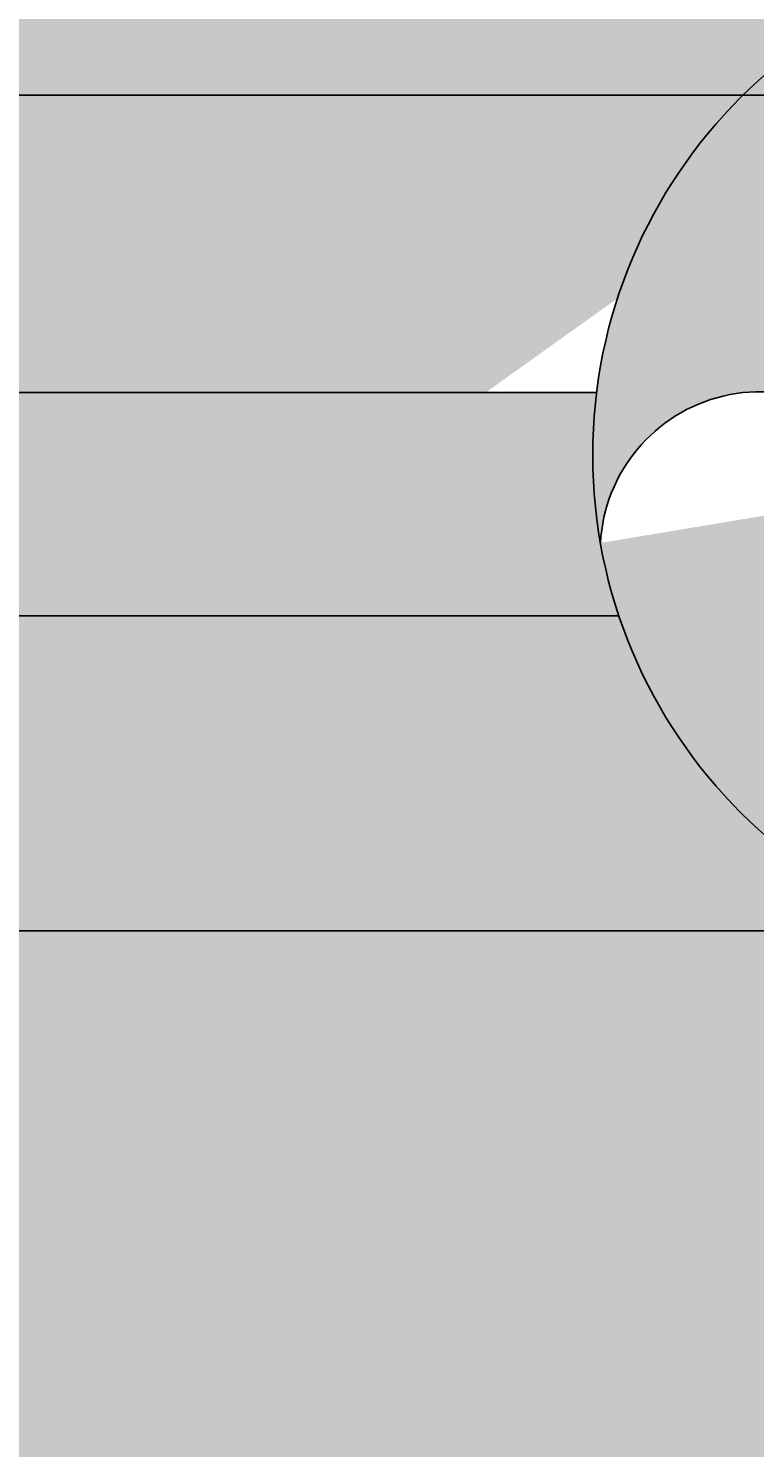
# Model space of a CAD drawing. Units: millimetres. Extents: x -22994 to 29398, y -19990 to 20176.
# Tile 114 of 135: x 204 to 220, y 124 to 156. Entities that reach past the tile are written whole.
import ezdxf

# ---------------------------------------------------------------- set-up
doc = ezdxf.new("R2010")
doc.units = ezdxf.units.MM
doc.header["$MEASUREMENT"] = 0
for name, color, linetype, lineweight in [('M-DIMS', 2, 'Continuous', 18), ('M-EQPM', 7, 'Continuous', 25), ('M-EQPM-PATT', 7, 'Continuous', 18)]:
    doc.layers.add(name, color=color, linetype=linetype, lineweight=lineweight)
doc.styles.get("Standard").update_dxf_attribs({"font": 'arial.ttf'})
doc.dimstyles.get("Standard").update_dxf_attribs({"dimtxt": 0.18, "dimasz": 10000, "dimexe": 0.18, "dimexo": 0.0625, "dimgap": 0.09, "dimtad": 0, "dimtih": 1, "dimtoh": 1, "dimdec": 0, "dimzin": 0, "dimdsep": 46, "dimtxsty": 'Standard', "dimcen": 0.09, "dimadec": 0, "dimazin": 0, "dimtfac": 1, "dimtdec": 0, "dimtofl": 0, "dimtmove": 0, "dimatfit": 3, "dimfxl": 1, "dimtolj": 1, "dimtzin": 0, "dimlwd": 30, "dimarcsym": 0})

# ---------------------------------------------------------------- blocks, each defined once
blk = doc.blocks.new('*D2')
at = {"layer": 'Defpoints', "color": 0, "transparency": 16777216}
for p in [(6.677, 10.271), (290.852, 10.271), (290.852, -5.079)]:
    blk.add_point(p, dxfattribs=at)
at = {"layer": 'M-DIMS', "color": 0, "lineweight": -2, "transparency": 16777216}
for p, q in [((6.677, 10.209), (6.677, -5.259)), ((290.852, 10.209), (290.852, -5.259))]:
    blk.add_line(p, q, dxfattribs=at)
at = {"layer": 'M-DIMS', "color": 0, "lineweight": 30, "transparency": 16777216}
for p, q in [((-9993.323, -5.079), (-19993.323, -5.079)), ((10290.852, -5.079), (20290.852, -5.079))]:
    blk.add_line(p, q, dxfattribs=at)
at = {"layer": 'M-DIMS', "color": 0, "transparency": 16777216}
for points in [[(-9993.323, 1661.588), (-9993.323, -1671.745), (6.677, -5.079)], [(10290.852, 1661.588), (10290.852, -1671.745), (290.852, -5.079)]]:
    blk.add_solid(points, dxfattribs=at)
at = {"layer": 'M-DIMS', "color": 0, "transparency": 16777216, "insert": (148.765, -5.079), "char_height": 0.18, "attachment_point": 5}
blk.add_mtext('\\A1;284.2', dxfattribs=at)
blk = doc.blocks.new('*D3')
at = {"layer": 'Defpoints', "color": 0, "transparency": 16777216}
for p in [(110.265, 204.165), (110.265, 176.366), (95.833, 127.967)]:
    blk.add_point(p, dxfattribs=at)
at = {"layer": 'M-DIMS', "color": 0, "lineweight": 30, "transparency": 16777216}
for p, q in [((-9904.167, 204.165), (-19904.167, 204.165)), ((10110.265, 204.165), (20110.265, 204.165))]:
    blk.add_line(p, q, dxfattribs=at)
at = {"layer": 'M-DIMS', "color": 0, "lineweight": -2, "transparency": 16777216}
for p, q in [((95.833, 128.03), (95.833, 204.345)), ((110.265, 176.429), (110.265, 204.345))]:
    blk.add_line(p, q, dxfattribs=at)
at = {"layer": 'M-DIMS', "color": 0, "transparency": 16777216}
for points in [[(-9904.167, 1870.832), (-9904.167, -1462.501), (95.833, 204.165)], [(10110.265, 1870.832), (10110.265, -1462.501), (110.265, 204.165)]]:
    blk.add_solid(points, dxfattribs=at)
at = {"layer": 'M-DIMS', "color": 0, "transparency": 16777216, "insert": (103.049, 204.165), "char_height": 0.18, "attachment_point": 5}
blk.add_mtext('\\A1;14.432', dxfattribs=at)
blk = doc.blocks.new('*D4')
at = {"layer": 'Defpoints', "color": 0, "transparency": 16777216}
for p in [(116.265, 204.165), (110.265, 176.366), (116.265, 176.366)]:
    blk.add_point(p, dxfattribs=at)
at = {"layer": 'M-DIMS', "color": 0, "lineweight": 30, "transparency": 16777216}
for p, q in [((-9889.735, 204.165), (-19889.735, 204.165)), ((10116.265, 204.165), (20116.265, 204.165))]:
    blk.add_line(p, q, dxfattribs=at)
at = {"layer": 'M-DIMS', "color": 0, "lineweight": -2, "transparency": 16777216}
for p, q in [((110.265, 176.429), (110.265, 204.345)), ((116.265, 176.429), (116.265, 204.345))]:
    blk.add_line(p, q, dxfattribs=at)
at = {"layer": 'M-DIMS', "color": 0, "transparency": 16777216}
for points in [[(-9889.735, 1870.832), (-9889.735, -1462.501), (110.265, 204.165)], [(10116.265, 1870.832), (10116.265, -1462.501), (116.265, 204.165)]]:
    blk.add_solid(points, dxfattribs=at)
at = {"layer": 'M-DIMS', "color": 0, "transparency": 16777216, "insert": (113.265, 204.165), "char_height": 0.18, "attachment_point": 5}
blk.add_mtext('\\A1;6', dxfattribs=at)
blk = doc.blocks.new('*D5')
at = {"layer": 'Defpoints', "color": 0, "transparency": 16777216}
for p in [(181.265, 204.165), (116.265, 176.366), (181.265, 176.366)]:
    blk.add_point(p, dxfattribs=at)
at = {"layer": 'M-DIMS', "color": 0, "lineweight": 30, "transparency": 16777216}
for p, q in [((-9883.735, 204.165), (-19883.735, 204.165)), ((10181.265, 204.165), (20181.265, 204.165))]:
    blk.add_line(p, q, dxfattribs=at)
at = {"layer": 'M-DIMS', "color": 0, "lineweight": -2, "transparency": 16777216}
for p, q in [((116.265, 176.429), (116.265, 204.345)), ((181.265, 176.429), (181.265, 204.345))]:
    blk.add_line(p, q, dxfattribs=at)
at = {"layer": 'M-DIMS', "color": 0, "transparency": 16777216}
for points in [[(-9883.735, 1870.832), (-9883.735, -1462.501), (116.265, 204.165)], [(10181.265, 1870.832), (10181.265, -1462.501), (181.265, 204.165)]]:
    blk.add_solid(points, dxfattribs=at)
at = {"layer": 'M-DIMS', "color": 0, "transparency": 16777216, "insert": (148.765, 204.165), "char_height": 0.18, "attachment_point": 5}
blk.add_mtext('\\A1;65', dxfattribs=at)
blk = doc.blocks.new('*D6')
at = {"layer": 'Defpoints', "color": 0, "transparency": 16777216}
for p in [(187.265, 204.165), (181.265, 176.366), (187.265, 176.366)]:
    blk.add_point(p, dxfattribs=at)
at = {"layer": 'M-DIMS', "color": 0, "lineweight": 30, "transparency": 16777216}
for p, q in [((-9818.735, 204.165), (-19818.735, 204.165)), ((10187.265, 204.165), (20187.265, 204.165))]:
    blk.add_line(p, q, dxfattribs=at)
at = {"layer": 'M-DIMS', "color": 0, "lineweight": -2, "transparency": 16777216}
for p, q in [((181.265, 176.429), (181.265, 204.345)), ((187.265, 176.429), (187.265, 204.345))]:
    blk.add_line(p, q, dxfattribs=at)
at = {"layer": 'M-DIMS', "color": 0, "transparency": 16777216}
for points in [[(-9818.735, 1870.832), (-9818.735, -1462.501), (181.265, 204.165)], [(10187.265, 1870.832), (10187.265, -1462.501), (187.265, 204.165)]]:
    blk.add_solid(points, dxfattribs=at)
at = {"layer": 'M-DIMS', "color": 0, "transparency": 16777216, "insert": (184.265, 204.165), "char_height": 0.18, "attachment_point": 5}
blk.add_mtext('\\A1;6', dxfattribs=at)
blk = doc.blocks.new('*D7')
at = {"layer": 'Defpoints', "color": 0, "transparency": 16777216}
for p in [(201.697, 204.165), (187.265, 176.366), (201.697, 127.967)]:
    blk.add_point(p, dxfattribs=at)
at = {"layer": 'M-DIMS', "color": 0, "lineweight": 30, "transparency": 16777216}
for p, q in [((-9812.735, 204.165), (-19812.735, 204.165)), ((10201.697, 204.165), (20201.697, 204.165))]:
    blk.add_line(p, q, dxfattribs=at)
at = {"layer": 'M-DIMS', "color": 0, "lineweight": -2, "transparency": 16777216}
for p, q in [((187.265, 176.429), (187.265, 204.345)), ((201.697, 128.03), (201.697, 204.345))]:
    blk.add_line(p, q, dxfattribs=at)
at = {"layer": 'M-DIMS', "color": 0, "transparency": 16777216}
for points in [[(-9812.735, 1870.832), (-9812.735, -1462.501), (187.265, 204.165)], [(10201.697, 1870.832), (10201.697, -1462.501), (201.697, 204.165)]]:
    blk.add_solid(points, dxfattribs=at)
at = {"layer": 'M-DIMS', "color": 0, "transparency": 16777216, "insert": (194.481, 204.165), "char_height": 0.18, "attachment_point": 5}
blk.add_mtext('\\A1;14.432', dxfattribs=at)
blk = doc.blocks.new('*D8')
at = {"layer": 'Defpoints', "color": 0, "transparency": 16777216}
for p in [(227.648, 204.165), (227.648, 146.73), (201.697, 127.967)]:
    blk.add_point(p, dxfattribs=at)
at = {"layer": 'M-DIMS', "color": 0, "lineweight": 30, "transparency": 16777216}
for p, q in [((-9798.303, 204.165), (-19798.303, 204.165)), ((10227.648, 204.165), (20227.648, 204.165))]:
    blk.add_line(p, q, dxfattribs=at)
at = {"layer": 'M-DIMS', "color": 0, "lineweight": -2, "transparency": 16777216}
for p, q in [((201.697, 128.03), (201.697, 204.345)), ((227.648, 146.792), (227.648, 204.345))]:
    blk.add_line(p, q, dxfattribs=at)
at = {"layer": 'M-DIMS', "color": 0, "transparency": 16777216}
for points in [[(-9798.303, 1870.832), (-9798.303, -1462.501), (201.697, 204.165)], [(10227.648, 1870.832), (10227.648, -1462.501), (227.648, 204.165)]]:
    blk.add_solid(points, dxfattribs=at)
at = {"layer": 'M-DIMS', "color": 0, "transparency": 16777216, "insert": (214.673, 204.165), "char_height": 0.18, "attachment_point": 5}
blk.add_mtext('\\A1;25.95', dxfattribs=at)
blk = doc.blocks.new('*D9')
at = {"layer": 'Defpoints', "color": 0, "transparency": 16777216}
for p in [(187.265, 176.366), (306.202, 176.366), (290.852, 10.271)]:
    blk.add_point(p, dxfattribs=at)
at = {"layer": 'M-DIMS', "color": 0, "lineweight": 30, "transparency": 16777216}
for p, q in [((306.202, 10176.366), (306.202, 20176.366)), ((306.202, -9989.729), (306.202, -19989.729))]:
    blk.add_line(p, q, dxfattribs=at)
at = {"layer": 'M-DIMS', "color": 0, "lineweight": -2, "transparency": 16777216}
for p, q in [((187.327, 176.366), (306.382, 176.366)), ((290.915, 10.271), (306.382, 10.271))]:
    blk.add_line(p, q, dxfattribs=at)
at = {"layer": 'M-DIMS', "color": 0, "transparency": 16777216}
for points in [[(-1360.465, 10176.366), (1972.869, 10176.366), (306.202, 176.366)], [(-1360.465, -9989.729), (1972.869, -9989.729), (306.202, 10.271)]]:
    blk.add_solid(points, dxfattribs=at)
at = {"layer": 'M-DIMS', "color": 0, "transparency": 16777216, "insert": (306.202, 93.319), "char_height": 0.18, "attachment_point": 5}
blk.add_mtext('\\A1;166.1', dxfattribs=at)
blk = doc.blocks.new('*D10')
at = {"layer": 'Defpoints', "color": 0, "transparency": 16777216}
for p in [(125.65, 136.071), (133.346, 136.071), (133.346, -5.079)]:
    blk.add_point(p, dxfattribs=at)
at = {"layer": 'M-DIMS', "color": 0, "lineweight": -2, "transparency": 16777216}
for p, q in [((125.65, 136.009), (125.65, -5.259)), ((133.346, 136.009), (133.346, -5.259))]:
    blk.add_line(p, q, dxfattribs=at)
at = {"layer": 'M-DIMS', "color": 0, "lineweight": 30, "transparency": 16777216}
for p, q in [((-9874.35, -5.079), (-19874.35, -5.079)), ((10133.346, -5.079), (20133.346, -5.079))]:
    blk.add_line(p, q, dxfattribs=at)
at = {"layer": 'M-DIMS', "color": 0, "transparency": 16777216}
for points in [[(-9874.35, 1661.588), (-9874.35, -1671.745), (125.65, -5.079)], [(10133.346, 1661.588), (10133.346, -1671.745), (133.346, -5.079)]]:
    blk.add_solid(points, dxfattribs=at)
at = {"layer": 'M-DIMS', "color": 0, "transparency": 16777216, "insert": (129.498, -5.079), "char_height": 0.18, "attachment_point": 5}
blk.add_mtext('\\A1;7.696', dxfattribs=at)
blk = doc.blocks.new('*D11')
at = {"layer": 'Defpoints', "color": 0, "transparency": 16777216}
for p in [(133.346, 136.071), (135.65, 136.071), (135.65, -5.079)]:
    blk.add_point(p, dxfattribs=at)
at = {"layer": 'M-DIMS', "color": 0, "lineweight": -2, "transparency": 16777216}
for p, q in [((133.346, 136.009), (133.346, -5.259)), ((135.65, 136.009), (135.65, -5.259))]:
    blk.add_line(p, q, dxfattribs=at)
at = {"layer": 'M-DIMS', "color": 0, "lineweight": 30, "transparency": 16777216}
for p, q in [((-9866.654, -5.079), (-19866.654, -5.079)), ((10135.65, -5.079), (20135.65, -5.079))]:
    blk.add_line(p, q, dxfattribs=at)
at = {"layer": 'M-DIMS', "color": 0, "transparency": 16777216}
for points in [[(-9866.654, 1661.588), (-9866.654, -1671.745), (133.346, -5.079)], [(10135.65, 1661.588), (10135.65, -1671.745), (135.65, -5.079)]]:
    blk.add_solid(points, dxfattribs=at)
at = {"layer": 'M-DIMS', "color": 0, "transparency": 16777216, "insert": (134.498, -5.079), "char_height": 0.18, "attachment_point": 5}
blk.add_mtext('\\A1;2.304', dxfattribs=at)
blk = doc.blocks.new('*D12')
at = {"layer": 'Defpoints', "color": 0, "transparency": 16777216}
for p in [(135.65, 136.071), (145.65, 136.071), (145.65, -5.079)]:
    blk.add_point(p, dxfattribs=at)
at = {"layer": 'M-DIMS', "color": 0, "lineweight": -2, "transparency": 16777216}
for p, q in [((135.65, 136.009), (135.65, -5.259)), ((145.65, 136.009), (145.65, -5.259))]:
    blk.add_line(p, q, dxfattribs=at)
at = {"layer": 'M-DIMS', "color": 0, "lineweight": 30, "transparency": 16777216}
for p, q in [((-9864.35, -5.079), (-19864.35, -5.079)), ((10145.65, -5.079), (20145.65, -5.079))]:
    blk.add_line(p, q, dxfattribs=at)
at = {"layer": 'M-DIMS', "color": 0, "transparency": 16777216}
for points in [[(-9864.35, 1661.588), (-9864.35, -1671.745), (135.65, -5.079)], [(10145.65, 1661.588), (10145.65, -1671.745), (145.65, -5.079)]]:
    blk.add_solid(points, dxfattribs=at)
at = {"layer": 'M-DIMS', "color": 0, "transparency": 16777216, "insert": (140.65, -5.079), "char_height": 0.18, "attachment_point": 5}
blk.add_mtext('\\A1;10', dxfattribs=at)
blk = doc.blocks.new('*D13')
at = {"layer": 'Defpoints', "color": 0, "transparency": 16777216}
for p in [(145.65, 136.071), (155.65, 136.071), (155.65, -5.079)]:
    blk.add_point(p, dxfattribs=at)
at = {"layer": 'M-DIMS', "color": 0, "lineweight": -2, "transparency": 16777216}
for p, q in [((145.65, 136.009), (145.65, -5.259)), ((155.65, 136.009), (155.65, -5.259))]:
    blk.add_line(p, q, dxfattribs=at)
at = {"layer": 'M-DIMS', "color": 0, "lineweight": 30, "transparency": 16777216}
for p, q in [((-9854.35, -5.079), (-19854.35, -5.079)), ((10155.65, -5.079), (20155.65, -5.079))]:
    blk.add_line(p, q, dxfattribs=at)
at = {"layer": 'M-DIMS', "color": 0, "transparency": 16777216}
for points in [[(-9854.35, 1661.588), (-9854.35, -1671.745), (145.65, -5.079)], [(10155.65, 1661.588), (10155.65, -1671.745), (155.65, -5.079)]]:
    blk.add_solid(points, dxfattribs=at)
at = {"layer": 'M-DIMS', "color": 0, "transparency": 16777216, "insert": (150.65, -5.079), "char_height": 0.18, "attachment_point": 5}
blk.add_mtext('\\A1;10', dxfattribs=at)
blk = doc.blocks.new('*D14')
at = {"layer": 'Defpoints', "color": 0, "transparency": 16777216}
for p in [(155.65, 136.071), (165.65, 136.071), (165.65, -5.079)]:
    blk.add_point(p, dxfattribs=at)
at = {"layer": 'M-DIMS', "color": 0, "lineweight": -2, "transparency": 16777216}
for p, q in [((155.65, 136.009), (155.65, -5.259)), ((165.65, 136.009), (165.65, -5.259))]:
    blk.add_line(p, q, dxfattribs=at)
at = {"layer": 'M-DIMS', "color": 0, "lineweight": 30, "transparency": 16777216}
for p, q in [((-9844.35, -5.079), (-19844.35, -5.079)), ((10165.65, -5.079), (20165.65, -5.079))]:
    blk.add_line(p, q, dxfattribs=at)
at = {"layer": 'M-DIMS', "color": 0, "transparency": 16777216}
for points in [[(-9844.35, 1661.588), (-9844.35, -1671.745), (155.65, -5.079)], [(10165.65, 1661.588), (10165.65, -1671.745), (165.65, -5.079)]]:
    blk.add_solid(points, dxfattribs=at)
at = {"layer": 'M-DIMS', "color": 0, "transparency": 16777216, "insert": (160.65, -5.079), "char_height": 0.18, "attachment_point": 5}
blk.add_mtext('\\A1;10', dxfattribs=at)
blk = doc.blocks.new('*D15')
at = {"layer": 'Defpoints', "color": 0, "transparency": 16777216}
for p in [(173.346, 154.788), (173.346, 136.071), (306.202, 136.071)]:
    blk.add_point(p, dxfattribs=at)
at = {"layer": 'M-DIMS', "color": 0, "lineweight": 30, "transparency": 16777216}
for p, q in [((306.202, 10154.788), (306.202, 20154.788)), ((306.202, -9863.929), (306.202, -19863.929))]:
    blk.add_line(p, q, dxfattribs=at)
at = {"layer": 'M-DIMS', "color": 0, "lineweight": -2, "transparency": 16777216}
for p, q in [((173.408, 154.788), (306.382, 154.788)), ((173.408, 136.071), (306.382, 136.071))]:
    blk.add_line(p, q, dxfattribs=at)
at = {"layer": 'M-DIMS', "color": 0, "transparency": 16777216}
for points in [[(-1360.465, 10154.788), (1972.869, 10154.788), (306.202, 154.788)], [(-1360.465, -9863.929), (1972.869, -9863.929), (306.202, 136.071)]]:
    blk.add_solid(points, dxfattribs=at)
at = {"layer": 'M-DIMS', "color": 0, "transparency": 16777216, "insert": (306.202, 145.43), "char_height": 0.18, "attachment_point": 5}
blk.add_mtext('\\A1;18.717', dxfattribs=at)
blk = doc.blocks.new('*D16')
at = {"layer": 'Defpoints', "color": 0, "transparency": 16777216}
for p in [(120.17, 204.165), (110.466, 48.035), (120.17, 48.035)]:
    blk.add_point(p, dxfattribs=at)
at = {"layer": 'M-DIMS', "color": 0, "lineweight": 30, "transparency": 16777216}
for p, q in [((-9889.534, 204.165), (-19889.534, 204.165)), ((10120.17, 204.165), (20120.17, 204.165))]:
    blk.add_line(p, q, dxfattribs=at)
at = {"layer": 'M-DIMS', "color": 0, "lineweight": -2, "transparency": 16777216}
for p, q in [((110.466, 48.097), (110.466, 204.345)), ((120.17, 48.097), (120.17, 204.345))]:
    blk.add_line(p, q, dxfattribs=at)
at = {"layer": 'M-DIMS', "color": 0, "transparency": 16777216}
for points in [[(-9889.534, 1870.832), (-9889.534, -1462.501), (110.466, 204.165)], [(10120.17, 1870.832), (10120.17, -1462.501), (120.17, 204.165)]]:
    blk.add_solid(points, dxfattribs=at)
at = {"layer": 'M-DIMS', "color": 0, "transparency": 16777216, "insert": (115.318, 204.165), "char_height": 0.18, "attachment_point": 5}
blk.add_mtext('\\A1;9.704', dxfattribs=at)
blk = doc.blocks.new('*D17')
at = {"layer": 'Defpoints', "color": 0, "transparency": 16777216}
for p in [(126.17, 204.165), (120.17, 48.035), (126.17, 48.035)]:
    blk.add_point(p, dxfattribs=at)
at = {"layer": 'M-DIMS', "color": 0, "lineweight": 30, "transparency": 16777216}
for p, q in [((-9879.83, 204.165), (-19879.83, 204.165)), ((10126.17, 204.165), (20126.17, 204.165))]:
    blk.add_line(p, q, dxfattribs=at)
at = {"layer": 'M-DIMS', "color": 0, "lineweight": -2, "transparency": 16777216}
for p, q in [((120.17, 48.097), (120.17, 204.345)), ((126.17, 48.097), (126.17, 204.345))]:
    blk.add_line(p, q, dxfattribs=at)
at = {"layer": 'M-DIMS', "color": 0, "transparency": 16777216}
for points in [[(-9879.83, 1870.832), (-9879.83, -1462.501), (120.17, 204.165)], [(10126.17, 1870.832), (10126.17, -1462.501), (126.17, 204.165)]]:
    blk.add_solid(points, dxfattribs=at)
at = {"layer": 'M-DIMS', "color": 0, "transparency": 16777216, "insert": (123.17, 204.165), "char_height": 0.18, "attachment_point": 5}
blk.add_mtext('\\A1;6', dxfattribs=at)
blk = doc.blocks.new('*D18')
at = {"layer": 'Defpoints', "color": 0, "transparency": 16777216}
for p in [(132.17, 204.165), (126.17, 48.035), (132.17, 48.035)]:
    blk.add_point(p, dxfattribs=at)
at = {"layer": 'M-DIMS', "color": 0, "lineweight": 30, "transparency": 16777216}
for p, q in [((-9873.83, 204.165), (-19873.83, 204.165)), ((10132.17, 204.165), (20132.17, 204.165))]:
    blk.add_line(p, q, dxfattribs=at)
at = {"layer": 'M-DIMS', "color": 0, "lineweight": -2, "transparency": 16777216}
for p, q in [((126.17, 48.097), (126.17, 204.345)), ((132.17, 48.097), (132.17, 204.345))]:
    blk.add_line(p, q, dxfattribs=at)
at = {"layer": 'M-DIMS', "color": 0, "transparency": 16777216}
for points in [[(-9873.83, 1870.832), (-9873.83, -1462.501), (126.17, 204.165)], [(10132.17, 1870.832), (10132.17, -1462.501), (132.17, 204.165)]]:
    blk.add_solid(points, dxfattribs=at)
at = {"layer": 'M-DIMS', "color": 0, "transparency": 16777216, "insert": (129.17, 204.165), "char_height": 0.18, "attachment_point": 5}
blk.add_mtext('\\A1;6', dxfattribs=at)
blk = doc.blocks.new('*D19')
at = {"layer": 'Defpoints', "color": 0, "transparency": 16777216}
for p in [(138.17, 204.165), (132.17, 48.035), (138.17, 48.035)]:
    blk.add_point(p, dxfattribs=at)
at = {"layer": 'M-DIMS', "color": 0, "lineweight": 30, "transparency": 16777216}
for p, q in [((-9867.83, 204.165), (-19867.83, 204.165)), ((10138.17, 204.165), (20138.17, 204.165))]:
    blk.add_line(p, q, dxfattribs=at)
at = {"layer": 'M-DIMS', "color": 0, "lineweight": -2, "transparency": 16777216}
for p, q in [((132.17, 48.097), (132.17, 204.345)), ((138.17, 48.097), (138.17, 204.345))]:
    blk.add_line(p, q, dxfattribs=at)
at = {"layer": 'M-DIMS', "color": 0, "transparency": 16777216}
for points in [[(-9867.83, 1870.832), (-9867.83, -1462.501), (132.17, 204.165)], [(10138.17, 1870.832), (10138.17, -1462.501), (138.17, 204.165)]]:
    blk.add_solid(points, dxfattribs=at)
at = {"layer": 'M-DIMS', "color": 0, "transparency": 16777216, "insert": (135.17, 204.165), "char_height": 0.18, "attachment_point": 5}
blk.add_mtext('\\A1;6', dxfattribs=at)
blk = doc.blocks.new('*D20')
at = {"layer": 'Defpoints', "color": 0, "transparency": 16777216}
for p in [(144.17, 204.165), (138.17, 48.035), (144.17, 48.035)]:
    blk.add_point(p, dxfattribs=at)
at = {"layer": 'M-DIMS', "color": 0, "lineweight": 30, "transparency": 16777216}
for p, q in [((-9861.83, 204.165), (-19861.83, 204.165)), ((10144.17, 204.165), (20144.17, 204.165))]:
    blk.add_line(p, q, dxfattribs=at)
at = {"layer": 'M-DIMS', "color": 0, "lineweight": -2, "transparency": 16777216}
for p, q in [((138.17, 48.097), (138.17, 204.345)), ((144.17, 48.097), (144.17, 204.345))]:
    blk.add_line(p, q, dxfattribs=at)
at = {"layer": 'M-DIMS', "color": 0, "transparency": 16777216}
for points in [[(-9861.83, 1870.832), (-9861.83, -1462.501), (138.17, 204.165)], [(10144.17, 1870.832), (10144.17, -1462.501), (144.17, 204.165)]]:
    blk.add_solid(points, dxfattribs=at)
at = {"layer": 'M-DIMS', "color": 0, "transparency": 16777216, "insert": (141.17, 204.165), "char_height": 0.18, "attachment_point": 5}
blk.add_mtext('\\A1;6', dxfattribs=at)
blk = doc.blocks.new('*D21')
at = {"layer": 'Defpoints', "color": 0, "transparency": 16777216}
for p in [(149.116, 204.165), (144.17, 48.035), (149.116, 48.035)]:
    blk.add_point(p, dxfattribs=at)
at = {"layer": 'M-DIMS', "color": 0, "lineweight": 30, "transparency": 16777216}
for p, q in [((-9855.83, 204.165), (-19855.83, 204.165)), ((10149.116, 204.165), (20149.116, 204.165))]:
    blk.add_line(p, q, dxfattribs=at)
at = {"layer": 'M-DIMS', "color": 0, "lineweight": -2, "transparency": 16777216}
for p, q in [((144.17, 48.097), (144.17, 204.345)), ((149.116, 48.097), (149.116, 204.345))]:
    blk.add_line(p, q, dxfattribs=at)
at = {"layer": 'M-DIMS', "color": 0, "transparency": 16777216}
for points in [[(-9855.83, 1870.832), (-9855.83, -1462.501), (144.17, 204.165)], [(10149.116, 1870.832), (10149.116, -1462.501), (149.116, 204.165)]]:
    blk.add_solid(points, dxfattribs=at)
at = {"layer": 'M-DIMS', "color": 0, "transparency": 16777216, "insert": (146.643, 204.165), "char_height": 0.18, "attachment_point": 5}
blk.add_mtext('\\A1;4.945', dxfattribs=at)
blk = doc.blocks.new('*D22')
at = {"layer": 'Defpoints', "color": 0, "transparency": 16777216}
for p in [(149.116, 30.99), (155.116, 30.99), (155.116, -5.079)]:
    blk.add_point(p, dxfattribs=at)
at = {"layer": 'M-DIMS', "color": 0, "lineweight": -2, "transparency": 16777216}
for p, q in [((149.116, 30.927), (149.116, -5.259)), ((155.116, 30.927), (155.116, -5.259))]:
    blk.add_line(p, q, dxfattribs=at)
at = {"layer": 'M-DIMS', "color": 0, "lineweight": 30, "transparency": 16777216}
for p, q in [((-9850.884, -5.079), (-19850.884, -5.079)), ((10155.116, -5.079), (20155.116, -5.079))]:
    blk.add_line(p, q, dxfattribs=at)
at = {"layer": 'M-DIMS', "color": 0, "transparency": 16777216}
for points in [[(-9850.884, 1661.588), (-9850.884, -1671.745), (149.116, -5.079)], [(10155.116, 1661.588), (10155.116, -1671.745), (155.116, -5.079)]]:
    blk.add_solid(points, dxfattribs=at)
at = {"layer": 'M-DIMS', "color": 0, "transparency": 16777216, "insert": (152.116, -5.079), "char_height": 0.18, "attachment_point": 5}
blk.add_mtext('\\A1;6', dxfattribs=at)
blk = doc.blocks.new('*D23')
at = {"layer": 'Defpoints', "color": 0, "transparency": 16777216}
for p in [(155.116, 30.99), (161.116, 30.99), (161.116, -5.079)]:
    blk.add_point(p, dxfattribs=at)
at = {"layer": 'M-DIMS', "color": 0, "lineweight": -2, "transparency": 16777216}
for p, q in [((155.116, 30.927), (155.116, -5.259)), ((161.116, 30.927), (161.116, -5.259))]:
    blk.add_line(p, q, dxfattribs=at)
at = {"layer": 'M-DIMS', "color": 0, "lineweight": 30, "transparency": 16777216}
for p, q in [((-9844.884, -5.079), (-19844.884, -5.079)), ((10161.116, -5.079), (20161.116, -5.079))]:
    blk.add_line(p, q, dxfattribs=at)
at = {"layer": 'M-DIMS', "color": 0, "transparency": 16777216}
for points in [[(-9844.884, 1661.588), (-9844.884, -1671.745), (155.116, -5.079)], [(10161.116, 1661.588), (10161.116, -1671.745), (161.116, -5.079)]]:
    blk.add_solid(points, dxfattribs=at)
at = {"layer": 'M-DIMS', "color": 0, "transparency": 16777216, "insert": (158.116, -5.079), "char_height": 0.18, "attachment_point": 5}
blk.add_mtext('\\A1;6', dxfattribs=at)
blk = doc.blocks.new('*D24')
at = {"layer": 'Defpoints', "color": 0, "transparency": 16777216}
for p in [(161.116, 30.99), (166.439, 30.99), (166.439, -5.079)]:
    blk.add_point(p, dxfattribs=at)
at = {"layer": 'M-DIMS', "color": 0, "lineweight": -2, "transparency": 16777216}
for p, q in [((161.116, 30.927), (161.116, -5.259)), ((166.439, 30.927), (166.439, -5.259))]:
    blk.add_line(p, q, dxfattribs=at)
at = {"layer": 'M-DIMS', "color": 0, "lineweight": 30, "transparency": 16777216}
for p, q in [((-9838.884, -5.079), (-19838.884, -5.079)), ((10166.439, -5.079), (20166.439, -5.079))]:
    blk.add_line(p, q, dxfattribs=at)
at = {"layer": 'M-DIMS', "color": 0, "transparency": 16777216}
for points in [[(-9838.884, 1661.588), (-9838.884, -1671.745), (161.116, -5.079)], [(10166.439, 1661.588), (10166.439, -1671.745), (166.439, -5.079)]]:
    blk.add_solid(points, dxfattribs=at)
at = {"layer": 'M-DIMS', "color": 0, "transparency": 16777216, "insert": (163.777, -5.079), "char_height": 0.18, "attachment_point": 5}
blk.add_mtext('\\A1;5.323', dxfattribs=at)
blk = doc.blocks.new('*D25')
at = {"layer": 'Defpoints', "color": 0, "transparency": 16777216}
for p in [(166.439, 30.99), (172.439, 30.99), (172.439, -5.079)]:
    blk.add_point(p, dxfattribs=at)
at = {"layer": 'M-DIMS', "color": 0, "lineweight": -2, "transparency": 16777216}
for p, q in [((166.439, 30.927), (166.439, -5.259)), ((172.439, 30.927), (172.439, -5.259))]:
    blk.add_line(p, q, dxfattribs=at)
at = {"layer": 'M-DIMS', "color": 0, "lineweight": 30, "transparency": 16777216}
for p, q in [((-9833.561, -5.079), (-19833.561, -5.079)), ((10172.439, -5.079), (20172.439, -5.079))]:
    blk.add_line(p, q, dxfattribs=at)
at = {"layer": 'M-DIMS', "color": 0, "transparency": 16777216}
for points in [[(-9833.561, 1661.588), (-9833.561, -1671.745), (166.439, -5.079)], [(10172.439, 1661.588), (10172.439, -1671.745), (172.439, -5.079)]]:
    blk.add_solid(points, dxfattribs=at)
at = {"layer": 'M-DIMS', "color": 0, "transparency": 16777216, "insert": (169.439, -5.079), "char_height": 0.18, "attachment_point": 5}
blk.add_mtext('\\A1;6', dxfattribs=at)
blk = doc.blocks.new('*D26')
at = {"layer": 'Defpoints', "color": 0, "transparency": 16777216}
for p in [(172.439, 30.99), (178.439, 30.99), (178.439, -5.079)]:
    blk.add_point(p, dxfattribs=at)
at = {"layer": 'M-DIMS', "color": 0, "lineweight": -2, "transparency": 16777216}
for p, q in [((172.439, 30.927), (172.439, -5.259)), ((178.439, 30.927), (178.439, -5.259))]:
    blk.add_line(p, q, dxfattribs=at)
at = {"layer": 'M-DIMS', "color": 0, "lineweight": 30, "transparency": 16777216}
for p, q in [((-9827.561, -5.079), (-19827.561, -5.079)), ((10178.439, -5.079), (20178.439, -5.079))]:
    blk.add_line(p, q, dxfattribs=at)
at = {"layer": 'M-DIMS', "color": 0, "transparency": 16777216}
for points in [[(-9827.561, 1661.588), (-9827.561, -1671.745), (172.439, -5.079)], [(10178.439, 1661.588), (10178.439, -1671.745), (178.439, -5.079)]]:
    blk.add_solid(points, dxfattribs=at)
at = {"layer": 'M-DIMS', "color": 0, "transparency": 16777216, "insert": (175.439, -5.079), "char_height": 0.18, "attachment_point": 5}
blk.add_mtext('\\A1;6', dxfattribs=at)
blk = doc.blocks.new('*D27')
at = {"layer": 'Defpoints', "color": 0, "transparency": 16777216}
for p in [(178.439, 30.99), (188.117, 30.99), (188.117, -5.079)]:
    blk.add_point(p, dxfattribs=at)
at = {"layer": 'M-DIMS', "color": 0, "lineweight": -2, "transparency": 16777216}
for p, q in [((178.439, 30.927), (178.439, -5.259)), ((188.117, 30.927), (188.117, -5.259))]:
    blk.add_line(p, q, dxfattribs=at)
at = {"layer": 'M-DIMS', "color": 0, "lineweight": 30, "transparency": 16777216}
for p, q in [((-9821.561, -5.079), (-19821.561, -5.079)), ((10188.117, -5.079), (20188.117, -5.079))]:
    blk.add_line(p, q, dxfattribs=at)
at = {"layer": 'M-DIMS', "color": 0, "transparency": 16777216}
for points in [[(-9821.561, 1661.588), (-9821.561, -1671.745), (178.439, -5.079)], [(10188.117, 1661.588), (10188.117, -1671.745), (188.117, -5.079)]]:
    blk.add_solid(points, dxfattribs=at)
at = {"layer": 'M-DIMS', "color": 0, "transparency": 16777216, "insert": (183.278, -5.079), "char_height": 0.18, "attachment_point": 5}
blk.add_mtext('\\A1;9.679', dxfattribs=at)
blk = doc.blocks.new('*D28')
at = {"layer": 'Defpoints', "color": 0, "transparency": 16777216}
for p in [(188.117, 48.035), (306.202, 48.035), (188.117, 30.99)]:
    blk.add_point(p, dxfattribs=at)
at = {"layer": 'M-DIMS', "color": 0, "lineweight": 30, "transparency": 16777216}
for p, q in [((306.202, 10048.035), (306.202, 20048.035)), ((306.202, -9969.01), (306.202, -19969.01))]:
    blk.add_line(p, q, dxfattribs=at)
at = {"layer": 'M-DIMS', "color": 0, "lineweight": -2, "transparency": 16777216}
for p, q in [((188.18, 48.035), (306.382, 48.035)), ((188.18, 30.99), (306.382, 30.99))]:
    blk.add_line(p, q, dxfattribs=at)
at = {"layer": 'M-DIMS', "color": 0, "transparency": 16777216}
for points in [[(-1360.465, 10048.035), (1972.869, 10048.035), (306.202, 48.035)], [(-1360.465, -9969.01), (1972.869, -9969.01), (306.202, 30.99)]]:
    blk.add_solid(points, dxfattribs=at)
at = {"layer": 'M-DIMS', "color": 0, "transparency": 16777216, "insert": (306.202, 39.512), "char_height": 0.18, "attachment_point": 5}
blk.add_mtext('\\A1;17.045', dxfattribs=at)
blk = doc.blocks.new('*D29')
at = {"layer": 'Defpoints', "color": 0, "transparency": 16777216}
for p in [(36.801, 80.045), (64.03, 80.045)]:
    blk.add_point(p, dxfattribs=at)
at = {"layer": 'M-DIMS', "color": 0, "lineweight": -2, "transparency": 16777216}
for p, q in [((50.415, 79.955), (50.415, 80.135)), ((50.325, 80.045), (50.505, 80.045))]:
    blk.add_line(p, q, dxfattribs=at)
at = {"layer": 'M-DIMS', "color": 0, "lineweight": 30, "transparency": 16777216}
blk.add_line((20064.03, 80.03), (10064.03, 80.038), dxfattribs=at)
at = {"layer": 'M-DIMS', "color": 0, "transparency": 16777216}
blk.add_solid([(10064.031, 1746.704), (10064.028, -1586.629), (64.03, 80.045)], dxfattribs=at)
at = {"layer": 'M-DIMS', "color": 0, "transparency": 16777216, "insert": (20064.521, 80.03), "char_height": 0.18, "attachment_point": 5}
blk.add_mtext('\\A1;∅27.23', dxfattribs=at)
blk = doc.blocks.new('*D30')
at = {"layer": 'Defpoints', "color": 0, "transparency": 16777216}
for p in [(216.315, 146.729), (238.982, 146.73)]:
    blk.add_point(p, dxfattribs=at)
at = {"layer": 'M-DIMS', "color": 0, "lineweight": 30, "transparency": 16777216}
blk.add_line((20238.982, 147.496), (10238.982, 147.113), dxfattribs=at)
at = {"layer": 'M-DIMS', "color": 0, "lineweight": -2, "transparency": 16777216}
for p, q in [((227.558, 146.73), (227.738, 146.73)), ((227.648, 146.64), (227.648, 146.82))]:
    blk.add_line(p, q, dxfattribs=at)
at = {"layer": 'M-DIMS', "color": 0, "transparency": 16777216}
blk.add_solid([(10238.918, 1813.78), (10239.046, -1519.554), (238.982, 146.73)], dxfattribs=at)
at = {"layer": 'M-DIMS', "color": 0, "transparency": 16777216, "insert": (20239.544, 147.496), "char_height": 0.18, "attachment_point": 5}
blk.add_mtext('\\A1;∅22.667', dxfattribs=at)
blk = doc.blocks.new('*D34')
at = {"layer": 'Defpoints', "color": 0, "transparency": 16777216}
for p in [(178.58, 122.895), (176.812, 121.128)]:
    blk.add_point(p, dxfattribs=at)
at = {"layer": 'M-DIMS', "color": 0, "lineweight": 30, "transparency": 16777216}
for p, q in [((14322.436, 14263.311), (7250.508, 7193.103)), ((24322.436, 14263.311), (14322.436, 14263.311))]:
    blk.add_line(p, q, dxfattribs=at)
at = {"layer": 'M-DIMS', "color": 0, "lineweight": -2, "transparency": 16777216}
for p, q in [((176.722, 121.128), (176.902, 121.128)), ((176.812, 121.038), (176.812, 121.218))]:
    blk.add_line(p, q, dxfattribs=at)
at = {"layer": 'M-DIMS', "color": 0, "transparency": 16777216}
blk.add_solid([(6072.14, 8371.758), (8428.876, 6014.448), (178.58, 122.895)], dxfattribs=at)
at = {"layer": 'M-DIMS', "color": 0, "transparency": 16777216, "insert": (24322.97, 14263.311), "char_height": 0.18, "attachment_point": 5}
blk.add_mtext('\\A1;6X R2.5', dxfattribs=at)
blk = doc.blocks.new('*D36')
at = {"layer": 'Defpoints', "color": 0, "transparency": 16777216}
for p in [(46.39, 31.303), (46.387, 26.593)]:
    blk.add_point(p, dxfattribs=at)
at = {"layer": 'M-DIMS', "color": 0, "lineweight": 30, "transparency": 16777216}
for p, q in [((57.15, 20031.301), (51.77, 10031.302)), ((10057.15, 20031.301), (57.15, 20031.301))]:
    blk.add_line(p, q, dxfattribs=at)
at = {"layer": 'M-DIMS', "color": 0, "lineweight": -2, "transparency": 16777216}
for p, q in [((46.299, 28.948), (46.479, 28.948)), ((46.389, 28.858), (46.389, 29.038))]:
    blk.add_line(p, q, dxfattribs=at)
at = {"layer": 'M-DIMS', "color": 0, "transparency": 16777216}
blk.add_solid([(-1614.896, 10032.199), (1718.436, 10030.405), (46.39, 31.303)], dxfattribs=at)
at = {"layer": 'M-DIMS', "color": 0, "transparency": 16777216, "insert": (10057.554, 20031.301), "char_height": 0.18, "attachment_point": 5}
blk.add_mtext('\\A1;∅4.71', dxfattribs=at)
blk = doc.blocks.new('*D37')
at = {"layer": 'Defpoints', "color": 0, "transparency": 16777216}
for p in [(54.834, 118.615), (59.494, 118.614)]:
    blk.add_point(p, dxfattribs=at)
at = {"layer": 'M-DIMS', "color": 0, "lineweight": -2, "transparency": 16777216}
for p, q in [((57.074, 118.614), (57.254, 118.614)), ((57.164, 118.524), (57.164, 118.704))]:
    blk.add_line(p, q, dxfattribs=at)
at = {"layer": 'M-DIMS', "color": 0, "lineweight": 30, "transparency": 16777216}
blk.add_line((20059.493, 116.253), (10059.494, 117.434), dxfattribs=at)
at = {"layer": 'M-DIMS', "color": 0, "transparency": 16777216}
blk.add_solid([(10059.69, 1784.1), (10059.297, -1549.233), (59.494, 118.614)], dxfattribs=at)
at = {"layer": 'M-DIMS', "color": 0, "transparency": 16777216, "insert": (20059.985, 116.253), "char_height": 0.18, "attachment_point": 5}
blk.add_mtext('\\A1;∅4.659', dxfattribs=at)

msp = doc.modelspace()

# ---------------------------------------------------------------- hatches: boundary and pattern name
at = {"layer": 'M-EQPM-PATT'}
h = msp.add_hatch(color=256, dxfattribs=at)
h.set_gradient(color1=(128, 128, 128), color2=(128, 128, 128), tint=1)
h.paths.add_polyline_path([(88.0003, 148.1301), (88.0003, 143.1301), (104.9278, 143.1301), (107.9269, 148.1301)])
h.paths.add_polyline_path([(189.6025, 148.1301), (192.6016, 143.1301), (216.9016, 143.1301, -0.0809736), (216.3148, 146.7296, -0.0309822), (216.4017, 148.1301)])
h.paths.add_polyline_path([(229.9653, 167.6546), (245.0476, 167.6546), (245.0476, 172.6546), (224.9653, 172.6546), (224.9653, 157.741, -0.1116822), (229.9653, 157.8239)])
h.paths.add_polyline_path([(36.3887, 21.6644), (36.3887, 16.6063), (56.3887, 16.6063), (56.3887, 21.6644)])
h = msp.add_hatch(color=256, dxfattribs=at)
h.set_gradient(color1=(0, 0, 255), color2=(244, 238, 81), tint=1, name='CYLINDER')
h.paths.add_polyline_path([(232.1163, 147.1148, 0.7475711), (238.8087, 148.7044, 0.2679492), (231.5183, 157.3821, -0.7475711), (229.5488, 150.7914, -0.2679492)])
h.paths.add_polyline_path([(216.3148, 146.7296, 0.0438131), (216.4882, 144.7547, -0.7475711), (223.1807, 146.3444, -0.0215046), (223.1641, 146.7296, -0.2450326), (225.081, 150.4062, 0.7475711), (220.3581, 155.4072, 0.2215353)])
h.paths.add_polyline_path([(234.9389, 138.0519, -0.7475711), (230.216, 143.053, -0.2679492), (225.7482, 142.6678, 0.7475711), (223.7786, 136.0771, 0.2679492)])

# ---------------------------------------------------------------- linework, layer by layer
at = {"layer": 'M-EQPM'}
for p, q in [((216.4017, 148.1301), (189.6025, 148.1301)), ((192.6016, 143.1301), (216.9016, 143.1301))]:
    msp.add_line(p, q, dxfattribs=at)
msp.add_circle((227.6485, 146.7296), 11.3336, dxfattribs=at)
msp.add_arc((220.069, 144.5622), 3.5859, 29.80022, 176.92313, dxfattribs=at)

# ---------------------------------------------------------------- dimensions: what is measured, and where the dimension line sits
at = {"layer": 'M-DIMS'}
for base, p1, p2, override, picture, middle in [((306.202, 176.3662), (290.852, 10.2713), (187.2647, 176.3662), {"dimdec": 1, "dimlfac": 1, "dimrnd": 0, "dimzin": 0, "dimdsep": 46, "dimlunit": 2}, '*D9', (306.202, 93.3187)), ((306.202, 136.0713), (173.3459, 154.788), (173.3459, 136.0713), {"dimdec": 3, "dimlfac": 1, "dimrnd": 0, "dimzin": 0, "dimdsep": 46, "dimlunit": 2}, '*D15', (306.202, 145.4297)), ((306.202, 48.0349), (188.1175, 30.9895), (188.1175, 48.0349), {"dimdec": 3, "dimlfac": 1, "dimrnd": 0, "dimzin": 0, "dimdsep": 46, "dimlunit": 2}, '*D28', (306.202, 39.5122))]:
    dim = msp.add_linear_dim(base=base, p1=p1, p2=p2, angle=90, dimstyle='Standard', override=override, dxfattribs=at)
    dim.commit()
    dim.dimension.update_dxf_attribs({"geometry": picture, "text_midpoint": middle})
for p1, p2, override, picture, middle in [((46.3875, 26.5934), (46.39, 31.3035), {"dimdec": 2, "dimlfac": 1, "dimrnd": 0, "dimzin": 0, "dimdsep": 46, "dimlunit": 2}, '*D36', (10057.5542, 20031.3006)), ((216.3148, 146.7291), (238.9821, 146.73), {"dimdec": 3, "dimlfac": 1, "dimrnd": 0, "dimzin": 0, "dimdsep": 46, "dimlunit": 2}, '*D30', (20238.9821, 147.4959))]:
    dim = msp.add_diameter_dim_2p(p1=p1, p2=p2, dimstyle='Standard', override=override, dxfattribs=at)
    dim.commit()
    dim.dimension.update_dxf_attribs({"geometry": picture, "text_midpoint": middle, "dimtype": 163})
dim = msp.add_radius_dim(center=(176.8123, 121.1277), mpoint=(178.5802, 122.8952), text='6X <>', dimstyle='Standard', override={"dimdec": 1, "dimlfac": 1, "dimrnd": 0, "dimzin": 0, "dimdsep": 46, "dimlunit": 2}, dxfattribs=at)
dim.commit()
dim.dimension.update_dxf_attribs({"geometry": '*D34', "text_midpoint": (24322.9703, 14263.3108)})
for base, p1, p2, override, picture, middle in [((110.2647, 204.1654), (95.8327, 127.967), (110.2647, 176.3662), {"dimdec": 3, "dimlfac": 1, "dimrnd": 0, "dimzin": 0, "dimdsep": 46, "dimlunit": 2}, '*D3', (103.0487, 204.1654)), ((116.2647, 204.1654), (110.2647, 176.3662), (116.2647, 176.3662), {"dimdec": 0, "dimlfac": 1, "dimrnd": 0, "dimzin": 0, "dimdsep": 46, "dimlunit": 2}, '*D4', (113.2647, 204.1654)), ((120.1702, 204.1654), (110.4658, 48.0349), (120.1702, 48.0349), {"dimdec": 3, "dimlfac": 1, "dimrnd": 0, "dimzin": 0, "dimdsep": 46, "dimlunit": 2}, '*D16', (115.318, 204.1654)), ((181.2647, 204.1654), (116.2647, 176.3662), (181.2647, 176.3662), {"dimdec": 0, "dimlfac": 1, "dimrnd": 0, "dimzin": 0, "dimdsep": 46, "dimlunit": 2}, '*D5', (148.7647, 204.1654)), ((126.1702, 204.1654), (120.1702, 48.0349), (126.1702, 48.0349), {"dimdec": 0, "dimlfac": 1, "dimrnd": 0, "dimzin": 0, "dimdsep": 46, "dimlunit": 2}, '*D17', (123.1702, 204.1654)), ((132.1702, 204.1654), (126.1702, 48.0349), (132.1702, 48.0349), {"dimdec": 0, "dimlfac": 1, "dimrnd": 0, "dimzin": 0, "dimdsep": 46, "dimlunit": 2}, '*D18', (129.1702, 204.1654)), ((138.1702, 204.1654), (132.1702, 48.0349), (138.1702, 48.0349), {"dimdec": 0, "dimlfac": 1, "dimrnd": 0, "dimzin": 0, "dimdsep": 46, "dimlunit": 2}, '*D19', (135.1702, 204.1654)), ((144.1702, 204.1654), (138.1702, 48.0349), (144.1702, 48.0349), {"dimdec": 0, "dimlfac": 1, "dimrnd": 0, "dimzin": 0, "dimdsep": 46, "dimlunit": 2}, '*D20', (141.1702, 204.1654)), ((149.11567, 204.16539), (144.17023, 48.03494), (149.11567, 48.03494), {"dimdec": 3, "dimlfac": 1, "dimrnd": 0, "dimzin": 0, "dimdsep": 46, "dimlunit": 2}, '*D21', (146.64295, 204.16539)), ((187.2647, 204.1654), (181.2647, 176.3662), (187.2647, 176.3662), {"dimdec": 0, "dimlfac": 1, "dimrnd": 0, "dimzin": 0, "dimdsep": 46, "dimlunit": 2}, '*D6', (184.2647, 204.1654)), ((201.6967, 204.1654), (187.2647, 176.3662), (201.6967, 127.967), {"dimdec": 3, "dimlfac": 1, "dimrnd": 0, "dimzin": 0, "dimdsep": 46, "dimlunit": 2}, '*D7', (194.4807, 204.1654)), ((227.6485, 204.1654), (201.6967, 127.967), (227.6485, 146.7296), {"dimdec": 2, "dimlfac": 1, "dimrnd": 0, "dimzin": 0, "dimdsep": 46, "dimlunit": 2}, '*D8', (214.6726, 204.1654)), ((290.852, -5.0787), (6.6773, 10.2713), (290.852, 10.2713), {"dimdec": 1, "dimlfac": 1, "dimrnd": 0, "dimzin": 0, "dimdsep": 46, "dimlunit": 2}, '*D2', (148.7647, -5.0787)), ((133.3459, -5.0787), (125.6498, 136.0713), (133.3459, 136.0713), {"dimdec": 3, "dimlfac": 1, "dimrnd": 0, "dimzin": 0, "dimdsep": 46, "dimlunit": 2}, '*D10', (129.4978, -5.0787)), ((135.6498, -5.0787), (133.3459, 136.0713), (135.6498, 136.0713), {"dimdec": 3, "dimlfac": 1, "dimrnd": 0, "dimzin": 0, "dimdsep": 46, "dimlunit": 2}, '*D11', (134.4978, -5.0787)), ((145.6498, -5.0787), (135.6498, 136.0713), (145.6498, 136.0713), {"dimdec": 0, "dimlfac": 1, "dimrnd": 0, "dimzin": 0, "dimdsep": 46, "dimlunit": 2}, '*D12', (140.6498, -5.0787)), ((155.6498, -5.0787), (145.6498, 136.0713), (155.6498, 136.0713), {"dimdec": 0, "dimlfac": 1, "dimrnd": 0, "dimzin": 0, "dimdsep": 46, "dimlunit": 2}, '*D13', (150.6498, -5.0787)), ((155.1157, -5.0787), (149.1157, 30.9895), (155.1157, 30.9895), {"dimdec": 0, "dimlfac": 1, "dimrnd": 0, "dimzin": 0, "dimdsep": 46, "dimlunit": 2}, '*D22', (152.1157, -5.0787)), ((161.1157, -5.0787), (155.1157, 30.9895), (161.1157, 30.9895), {"dimdec": 0, "dimlfac": 1, "dimrnd": 0, "dimzin": 0, "dimdsep": 46, "dimlunit": 2}, '*D23', (158.1157, -5.0787)), ((165.6498, -5.0787), (155.6498, 136.0713), (165.6498, 136.0713), {"dimdec": 0, "dimlfac": 1, "dimrnd": 0, "dimzin": 0, "dimdsep": 46, "dimlunit": 2}, '*D14', (160.6498, -5.0787)), ((166.4387, -5.0787), (161.1157, 30.9895), (166.4387, 30.9895), {"dimdec": 3, "dimlfac": 1, "dimrnd": 0, "dimzin": 0, "dimdsep": 46, "dimlunit": 2}, '*D24', (163.7772, -5.0787)), ((172.4387, -5.0787), (166.4387, 30.9895), (172.4387, 30.9895), {"dimdec": 0, "dimlfac": 1, "dimrnd": 0, "dimzin": 0, "dimdsep": 46, "dimlunit": 2}, '*D25', (169.4387, -5.0787)), ((178.4387, -5.0787), (172.4387, 30.9895), (178.4387, 30.9895), {"dimdec": 0, "dimlfac": 1, "dimrnd": 0, "dimzin": 0, "dimdsep": 46, "dimlunit": 2}, '*D26', (175.4387, -5.0787)), ((188.1175, -5.0787), (178.4387, 30.9895), (188.1175, 30.9895), {"dimdec": 3, "dimlfac": 1, "dimrnd": 0, "dimzin": 0, "dimdsep": 46, "dimlunit": 2}, '*D27', (183.2781, -5.0787))]:
    dim = msp.add_linear_dim(base=base, p1=p1, p2=p2, dimstyle='Standard', override=override, dxfattribs=at)
    dim.commit()
    dim.dimension.update_dxf_attribs({"geometry": picture, "text_midpoint": middle})
for p1, p2, override, picture, middle in [((54.8343, 118.6145), (59.4936, 118.614), {"dimdec": 3, "dimlfac": 1, "dimrnd": 0, "dimzin": 0, "dimdsep": 46, "dimlunit": 2}, '*D37', (20059.4934, 116.2531)), ((36.8006, 80.045), (64.0296, 80.045), {"dimdec": 2, "dimlfac": 1, "dimrnd": 0, "dimzin": 0, "dimdsep": 46, "dimlunit": 2}, '*D29', (20064.0296, 80.0303))]:
    dim = msp.add_diameter_dim_2p(p1=p1, p2=p2, dimstyle='Standard', override=override, dxfattribs=at)
    dim.commit()
    dim.dimension.update_dxf_attribs({"geometry": picture, "text_midpoint": middle})

doc.saveas('drawing.dxf')
